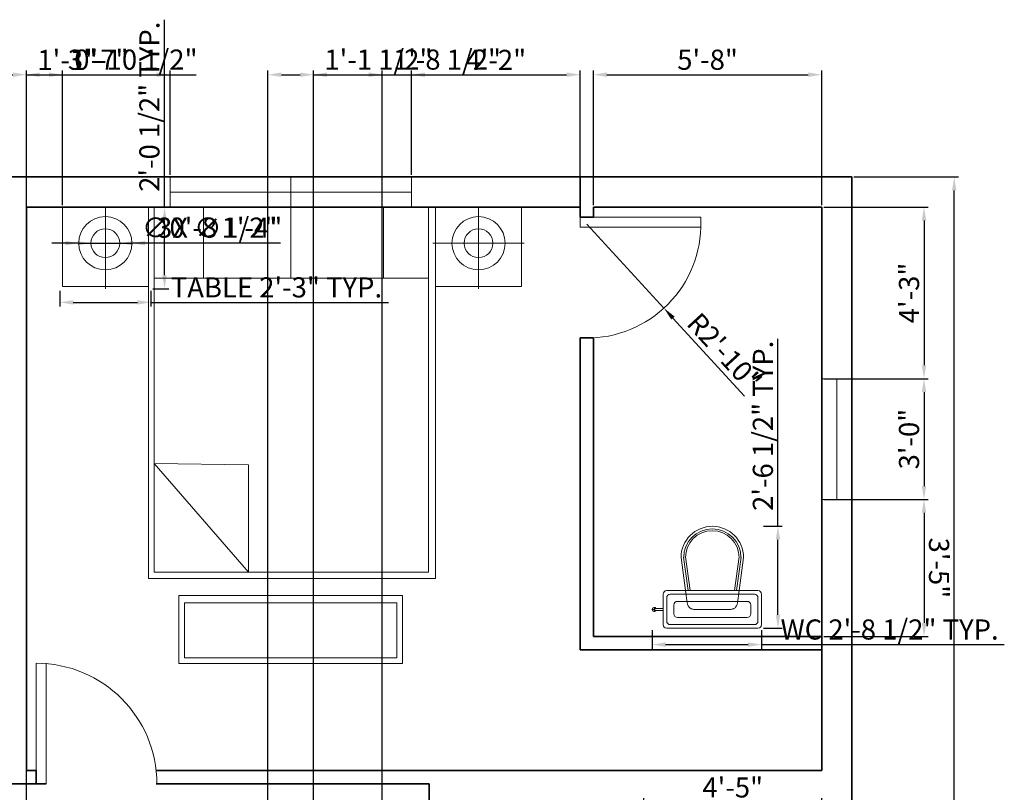
# Model space of a CAD drawing. Units: inches. Extents: x 1973 to 2661, y 1730 to 2412.
# Tile 5 of 5: x 2368 to 2661, y 2182 to 2412. Entities that reach past the tile are written whole.
import ezdxf

# ---------------------------------------------------------------- set-up
doc = ezdxf.new("R2010")
doc.units = ezdxf.units.IN
doc.linetypes.add('ACAD_ISO03W100', pattern=[30, 12, -18])
for name, color, linetype, lineweight in [('A-ANNO-DIMS', 2, 'Continuous', 18), ('A-DOOR', 3, 'Continuous', 18), ('A-FLOR-FIXT', 9, 'Continuous', 18), ('A-FLOR-FIXT-HIDN', 9, 'ACAD_ISO03W100', 13), ('A-FURN', 8, 'Continuous', 18), ('A-GLAZ', 4, 'Continuous', 18), ('A-WALL', 7, 'Continuous', 35)]:
    doc.layers.add(name, color=color, linetype=linetype, lineweight=lineweight)
doc.styles.get("Standard").update_dxf_attribs({"font": 'arial.ttf'})
doc.dimstyles.new('ISO-25', dxfattribs={"dimtxt": 6, "dimasz": 4, "dimexe": 1.25, "dimexo": 0.625, "dimtad": 1, "dimdec": 0, "dimrnd": 6, "dimlunit": 3, "dimtxsty": 'Standard', "dimcen": 2.5, "dimadec": 0, "dimazin": 0, "dimtfac": 1, "dimtdec": 0, "dimtmove": 0, "dimatfit": 3, "dimfxl": 1, "dimarcsym": 0})

# ---------------------------------------------------------------- blocks, each defined once
blk = doc.blocks.new('DOOR-36-SWING')
for p, q in [((0, 0), (0, 36)), ((0, 36), (0, 0)), ((3, 0), (3, 36)), ((0, 0), (3, 0))]:
    blk.add_line(p, q)
blk.add_arc((0, 0), 36, 0, 90)
blk = doc.blocks.new('WIN-72-TWO-LIGHT')
for p, q in [((0, 72), (9, 72)), ((0, 0), (0, 72)), ((4.5, 72), (4.5, 36)), ((9, 72), (9, 0)), ((4.5, 36), (0, 36)), ((0, 36), (9, 36)), ((4.5, 36), (4.5, 0)), ((9, 0), (0, 0))]:
    blk.add_line(p, q)
blk = doc.blocks.new('WC-TANK-PLAN')
for p, q in [((9.95, 11.2), (8.6, 21.07)), ((10.75, 11.2), (9.39, 21.19)), ((11.29, 11.2), (9.92, 21.26)), ((25.95, 21.26), (24.57, 11.2)), ((26.48, 21.19), (25.11, 11.2)), ((27.27, 21.07), (25.92, 11.2)), ((3.27, 1.07), (3.27, 10.13)), ((31.53, 11.2), (4.33, 11.2)), ((4.33, 2.13), (4.33, 9.07)), ((30.47, 10.13), (5.4, 10.13)), ((31.53, 2.13), (31.53, 9.07)), ((32.6, 1.07), (32.6, 10.13)), ((6.47, 4.27), (6.47, 6.93)), ((28.33, 8), (7.53, 8)), ((29.4, 4.27), (29.4, 6.93)), ((0.94, 5.6), (0.22, 5.6)), ((0.6, 5.33), (0.6, 5.87)), ((3.27, 5.87), (0.6, 5.87)), ((3.27, 5.33), (0.6, 5.33)), ((28.33, 3.2), (7.53, 3.2)), ((30.47, 1.07), (5.4, 1.07)), ((31.53, 0), (4.33, 0))]:
    blk.add_line(p, q)
for centre, radius, start, end in [((17.93, 21.07), 9.33, 0, 180), ((17.93, 21.07), 8.53, 0, 180), ((17.93, 21.07), 8, 0, 180), ((4.33, 10.13), 1.07, 90, 180), ((5.4, 9.07), 1.07, 90, 180), ((30.47, 9.07), 1.07, 0, 90), ((31.53, 10.13), 1.07, 0, 90), ((0.6, 5.6), 0.599, 26.4407, 333.5593), ((7.53, 6.93), 1.07, 90, 180), ((28.33, 6.93), 1.07, 0, 90), ((7.53, 4.27), 1.07, 180, 270), ((28.33, 4.27), 1.07, 270, 0), ((4.33, 1.07), 1.07, 180, 270), ((5.4, 2.13), 1.07, 180, 270), ((30.47, 2.13), 1.07, 270, 0), ((31.53, 1.07), 1.07, 270, 0)]:
    blk.add_arc(centre, radius, start, end)
blk = doc.blocks.new('BENCH-BED-END')
for p, q in [((0, 20.3), (0, 0)), ((66.64, 20.3), (0, 20.3)), ((1.73, 1.73), (1.73, 18.14)), ((1.73, 18.14), (64.92, 18.14)), ((64.92, 18.14), (64.92, 1.73)), ((66.64, 0), (66.64, 20.3)), ((64.92, 1.73), (1.73, 1.73)), ((0, 0), (66.64, 0))]:
    blk.add_line(p, q)
blk = doc.blocks.new('NIGHTSTAND-WITH-LAMP')
for p, q in [((0.77, 24.32), (0.77, 0.62)), ((13.58, 24.32, -15.39), (13.58, 0, -15.39)), ((27.15, 13.57, -15.39), (0, 13.57, -15.39)), ((0.77, 0.62), (26.42, 0.62))]:
    blk.add_line(p, q)
for radius in [7.93, 4.28]:
    blk.add_circle((13.58, 13.57, -15.39), radius)
blk = doc.blocks.new('*D22')
at = {"layer": 'A-ANNO-DIMS', "color": 0, "lineweight": -2, "transparency": 16777216}
for p, q in [((2556.52, 2230.17), (2556.52, 2224.65)), ((2589.12, 2230.17), (2589.12, 2224.65)), ((2560.52, 2225.9), (2585.12, 2225.9)), ((2589.12, 2225.9), (2661.47, 2225.9))]:
    blk.add_line(p, q, dxfattribs=at)
at = {"layer": 'A-ANNO-DIMS', "color": 0, "transparency": 16777216}
for points in [[(2560.52, 2226.57), (2560.52, 2225.24), (2556.52, 2225.9)], [(2585.12, 2226.57), (2585.12, 2225.24), (2589.12, 2225.9)]]:
    blk.add_solid(points, dxfattribs=at)
at = {"layer": 'Defpoints', "color": 0, "transparency": 16777216}
for p in [(2556.52, 2230.79), (2589.12, 2230.79), (2589.12, 2225.9)]:
    blk.add_point(p, dxfattribs=at)
at = {"layer": 'A-ANNO-DIMS', "color": 0, "transparency": 16777216, "insert": (2627.29, 2229.63), "char_height": 6, "attachment_point": 5}
blk.add_mtext('WC 2\'-8 1/2" TYP.', dxfattribs=at)
blk = doc.blocks.new('*D23')
at = {"layer": 'A-ANNO-DIMS', "color": 0, "lineweight": -2, "transparency": 16777216}
for p, q in [((2594.01, 2261.19), (2594.01, 2317.1)), ((2589.75, 2261.19), (2595.26, 2261.19)), ((2594.01, 2234.79), (2594.01, 2257.19)), ((2589.75, 2230.79), (2595.26, 2230.79))]:
    blk.add_line(p, q, dxfattribs=at)
at = {"layer": 'A-ANNO-DIMS', "color": 0, "transparency": 16777216}
for points in [[(2593.35, 2257.19), (2594.68, 2257.19), (2594.01, 2261.19)], [(2593.35, 2234.79), (2594.68, 2234.79), (2594.01, 2230.79)]]:
    blk.add_solid(points, dxfattribs=at)
at = {"layer": 'Defpoints', "color": 0, "transparency": 16777216}
for p in [(2589.12, 2261.19), (2594.01, 2261.19), (2589.12, 2230.79)]:
    blk.add_point(p, dxfattribs=at)
at = {"layer": 'A-ANNO-DIMS', "color": 0, "transparency": 16777216, "insert": (2590.29, 2291.15), "char_height": 6, "attachment_point": 5, "rotation": 90}
blk.add_mtext('2\'-6 1/2" TYP.', dxfattribs=at)
blk = doc.blocks.new('*D26')
at = {"layer": 'A-ANNO-DIMS', "color": 0, "lineweight": -2, "transparency": 16777216}
for p, q in [((2379.99, 2331.41), (2379.99, 2326.71)), ((2407.14, 2331.41), (2407.14, 2326.71)), ((2383.99, 2327.96), (2403.14, 2327.96)), ((2407.14, 2327.96), (2477.99, 2327.96))]:
    blk.add_line(p, q, dxfattribs=at)
at = {"layer": 'A-ANNO-DIMS', "color": 0, "transparency": 16777216}
for points in [[(2383.99, 2328.62), (2383.99, 2327.29), (2379.99, 2327.96)], [(2403.14, 2328.62), (2403.14, 2327.29), (2407.14, 2327.96)]]:
    blk.add_solid(points, dxfattribs=at)
at = {"layer": 'Defpoints', "color": 0, "transparency": 16777216}
for p in [(2379.99, 2332.03), (2407.14, 2332.03), (2407.14, 2327.96)]:
    blk.add_point(p, dxfattribs=at)
at = {"layer": 'A-ANNO-DIMS', "color": 0, "transparency": 16777216, "insert": (2444.56, 2331.65), "char_height": 6, "attachment_point": 5}
blk.add_mtext('TABLE 2\'-3" TYP.', dxfattribs=at)
blk = doc.blocks.new('*D27')
at = {"layer": 'A-ANNO-DIMS', "color": 0, "lineweight": -2, "transparency": 16777216}
for p, q in [((2411.21, 2356.35), (2411.21, 2412.26)), ((2407.76, 2356.35), (2412.46, 2356.35)), ((2411.21, 2336.03), (2411.21, 2352.35)), ((2407.76, 2332.03), (2412.46, 2332.03))]:
    blk.add_line(p, q, dxfattribs=at)
at = {"layer": 'A-ANNO-DIMS', "color": 0, "transparency": 16777216}
for points in [[(2410.54, 2352.35), (2411.87, 2352.35), (2411.21, 2356.35)], [(2410.54, 2336.03), (2411.87, 2336.03), (2411.21, 2332.03)]]:
    blk.add_solid(points, dxfattribs=at)
at = {"layer": 'Defpoints', "color": 0, "transparency": 16777216}
for p in [(2407.14, 2356.35), (2411.21, 2356.35), (2407.14, 2332.03)]:
    blk.add_point(p, dxfattribs=at)
at = {"layer": 'A-ANNO-DIMS', "color": 0, "transparency": 16777216, "insert": (2407.48, 2386.3), "char_height": 6, "attachment_point": 5, "rotation": 90}
blk.add_mtext('2\'-0 1/2" TYP.', dxfattribs=at)
blk = doc.blocks.new('*D31')
at = {"layer": 'A-ANNO-DIMS', "color": 0, "lineweight": -2, "transparency": 16777216}
for p, q in [((2616.67, 2365.35), (2647.79, 2365.35)), ((2646.54, 1769.35), (2646.54, 2361.35)), ((2616.67, 1765.35), (2647.79, 1765.35))]:
    blk.add_line(p, q, dxfattribs=at)
at = {"layer": 'A-ANNO-DIMS', "color": 0, "transparency": 16777216}
for points in [[(2645.88, 2361.35), (2647.21, 2361.35), (2646.54, 2365.35)], [(2645.88, 1769.35), (2647.21, 1769.35), (2646.54, 1765.35)]]:
    blk.add_solid(points, dxfattribs=at)
at = {"layer": 'Defpoints', "color": 0, "transparency": 16777216}
for p in [(2616.04, 2365.35), (2646.54, 2365.35), (2616.04, 1765.35)]:
    blk.add_point(p, dxfattribs=at)
at = {"layer": 'A-ANNO-DIMS', "color": 0, "transparency": 16777216, "insert": (2642.85, 2065.35), "char_height": 6, "attachment_point": 5, "rotation": 90}
blk.add_mtext('50\'-0"', dxfattribs=at)
blk = doc.blocks.new('*D37')
at = {"layer": 'A-ANNO-DIMS', "color": 0, "lineweight": -2, "transparency": 16777216}
for p, q in [((2370.04, 2356.98), (2370.04, 2397.1)), ((2374.04, 2395.85), (2408.84, 2395.85)), ((2412.84, 2365.96), (2412.84, 2397.1))]:
    blk.add_line(p, q, dxfattribs=at)
at = {"layer": 'A-ANNO-DIMS', "color": 0, "transparency": 16777216}
for points in [[(2374.04, 2396.52), (2374.04, 2395.18), (2370.04, 2395.85)], [(2408.84, 2396.52), (2408.84, 2395.18), (2412.84, 2395.85)]]:
    blk.add_solid(points, dxfattribs=at)
at = {"layer": 'Defpoints', "color": 0, "transparency": 16777216}
for p in [(2412.84, 2395.85), (2412.84, 2365.34), (2370.04, 2356.35)]:
    blk.add_point(p, dxfattribs=at)
at = {"layer": 'A-ANNO-DIMS', "color": 0, "transparency": 16777216, "insert": (2391.44, 2399.54), "char_height": 6, "attachment_point": 5}
blk.add_mtext('3\'-7"', dxfattribs=at)
blk = doc.blocks.new('*D38')
at = {"layer": 'A-ANNO-DIMS', "color": 0, "lineweight": -2, "transparency": 16777216}
for p, q in [((2484.84, 2365.96), (2484.84, 2397.1)), ((2488.84, 2395.85), (2531.04, 2395.85)), ((2535.04, 2356.98), (2535.04, 2397.1))]:
    blk.add_line(p, q, dxfattribs=at)
at = {"layer": 'A-ANNO-DIMS', "color": 0, "transparency": 16777216}
for points in [[(2488.84, 2396.52), (2488.84, 2395.18), (2484.84, 2395.85)], [(2531.04, 2396.52), (2531.04, 2395.18), (2535.04, 2395.85)]]:
    blk.add_solid(points, dxfattribs=at)
at = {"layer": 'Defpoints', "color": 0, "transparency": 16777216}
for p in [(2535.04, 2395.85), (2484.84, 2365.34), (2535.04, 2356.35)]:
    blk.add_point(p, dxfattribs=at)
at = {"layer": 'A-ANNO-DIMS', "color": 0, "transparency": 16777216, "insert": (2509.94, 2399.49), "char_height": 6, "attachment_point": 5}
blk.add_mtext('4\'-2"', dxfattribs=at)
blk = doc.blocks.new('*D39')
at = {"layer": 'A-ANNO-DIMS', "color": 0, "lineweight": -2, "transparency": 16777216}
for p, q in [((2539.04, 2356.98), (2539.04, 2397.1)), ((2543.04, 2395.85), (2603.04, 2395.85)), ((2607.04, 2356.98), (2607.04, 2397.1))]:
    blk.add_line(p, q, dxfattribs=at)
at = {"layer": 'A-ANNO-DIMS', "color": 0, "transparency": 16777216}
for points in [[(2543.04, 2396.52), (2543.04, 2395.18), (2539.04, 2395.85)], [(2603.04, 2396.52), (2603.04, 2395.18), (2607.04, 2395.85)]]:
    blk.add_solid(points, dxfattribs=at)
at = {"layer": 'Defpoints', "color": 0, "transparency": 16777216}
for p in [(2607.04, 2395.85), (2539.04, 2356.35), (2607.04, 2356.35)]:
    blk.add_point(p, dxfattribs=at)
at = {"layer": 'A-ANNO-DIMS', "color": 0, "transparency": 16777216, "insert": (2573.04, 2399.54), "char_height": 6, "attachment_point": 5}
blk.add_mtext('5\'-8"', dxfattribs=at)
blk = doc.blocks.new('*D50')
at = {"layer": 'A-ANNO-DIMS', "color": 0, "lineweight": -2, "transparency": 16777216}
for p, q in [((2607.66, 2269.19), (2638.79, 2269.2)), ((2637.54, 2265.2), (2637.54, 2232.36)), ((2607.67, 2228.35), (2638.79, 2228.36))]:
    blk.add_line(p, q, dxfattribs=at)
at = {"layer": 'A-ANNO-DIMS', "color": 0, "transparency": 16777216}
for points in [[(2638.2, 2265.2), (2636.87, 2265.2), (2637.54, 2269.2)], [(2638.21, 2232.36), (2636.88, 2232.36), (2637.54, 2228.36)]]:
    blk.add_solid(points, dxfattribs=at)
at = {"layer": 'Defpoints', "color": 0, "transparency": 16777216}
for p in [(2607.04, 2269.19), (2607.04, 2228.35), (2637.54, 2228.36)]:
    blk.add_point(p, dxfattribs=at)
at = {"layer": 'A-ANNO-DIMS', "color": 0, "transparency": 16777216, "insert": (2641.23, 2248.78), "char_height": 6, "attachment_point": 5, "rotation": 270.0074}
blk.add_mtext('3\'-5"', dxfattribs=at)
blk = doc.blocks.new('*D51')
at = {"layer": 'A-ANNO-DIMS', "color": 0, "lineweight": -2, "transparency": 16777216}
for p, q in [((2607.66, 2305.19), (2638.79, 2305.19)), ((2637.54, 2301.19), (2637.54, 2273.19)), ((2607.66, 2269.19), (2638.79, 2269.19))]:
    blk.add_line(p, q, dxfattribs=at)
at = {"layer": 'A-ANNO-DIMS', "color": 0, "transparency": 16777216}
for points in [[(2636.87, 2301.19), (2638.2, 2301.19), (2637.54, 2305.19)], [(2636.87, 2273.19), (2638.2, 2273.19), (2637.54, 2269.19)]]:
    blk.add_solid(points, dxfattribs=at)
at = {"layer": 'Defpoints', "color": 0, "transparency": 16777216}
for p in [(2607.04, 2305.19), (2607.04, 2269.19), (2637.54, 2269.19)]:
    blk.add_point(p, dxfattribs=at)
at = {"layer": 'A-ANNO-DIMS', "color": 0, "transparency": 16777216, "insert": (2633.85, 2287.19), "char_height": 6, "attachment_point": 5, "rotation": 90}
blk.add_mtext('3\'-0"', dxfattribs=at)
blk = doc.blocks.new('*D52')
at = {"layer": 'A-ANNO-DIMS', "color": 0, "lineweight": -2, "transparency": 16777216}
for p, q in [((2607.67, 2356.35), (2638.79, 2356.35)), ((2637.54, 2352.35), (2637.54, 2309.19)), ((2607.66, 2305.19), (2638.79, 2305.19))]:
    blk.add_line(p, q, dxfattribs=at)
at = {"layer": 'A-ANNO-DIMS', "color": 0, "transparency": 16777216}
for points in [[(2636.88, 2352.35), (2638.21, 2352.35), (2637.54, 2356.35)], [(2636.87, 2309.19), (2638.2, 2309.19), (2637.54, 2305.19)]]:
    blk.add_solid(points, dxfattribs=at)
at = {"layer": 'Defpoints', "color": 0, "transparency": 16777216}
for p in [(2607.04, 2356.35), (2607.04, 2305.19), (2637.54, 2305.19)]:
    blk.add_point(p, dxfattribs=at)
at = {"layer": 'A-ANNO-DIMS', "color": 0, "transparency": 16777216, "insert": (2633.85, 2330.77), "char_height": 6, "attachment_point": 5, "rotation": 89.9941}
blk.add_mtext('4\'-3"', dxfattribs=at)
blk = doc.blocks.new('*D63')
at = {"layer": 'A-ANNO-DIMS', "color": 0, "lineweight": -2, "transparency": 16777216}
for p, q in [((2554.04, 2148.98), (2554.04, 2180.1)), ((2558.04, 2178.85), (2603.04, 2178.85)), ((2607.04, 2148.98), (2607.04, 2180.1))]:
    blk.add_line(p, q, dxfattribs=at)
at = {"layer": 'A-ANNO-DIMS', "color": 0, "transparency": 16777216}
for points in [[(2558.04, 2179.52), (2558.04, 2178.18), (2554.04, 2178.85)], [(2603.04, 2179.52), (2603.04, 2178.18), (2607.04, 2178.85)]]:
    blk.add_solid(points, dxfattribs=at)
at = {"layer": 'Defpoints', "color": 0, "transparency": 16777216}
for p in [(2607.04, 2178.85), (2554.04, 2148.35), (2607.04, 2148.35)]:
    blk.add_point(p, dxfattribs=at)
at = {"layer": 'A-ANNO-DIMS', "color": 0, "transparency": 16777216, "insert": (2580.54, 2182.53), "char_height": 6, "attachment_point": 5}
blk.add_mtext('4\'-5"', dxfattribs=at)
blk = doc.blocks.new('*D67')
at = {"layer": 'A-ANNO-DIMS', "color": 0, "lineweight": -2, "transparency": 16777216}
for p, q in [((2455.64, 1843.98), (2455.64, 2397.1)), ((2459.64, 2395.85), (2472.06, 2395.85)), ((2476.06, 1843.98), (2476.06, 2397.1)), ((2476.06, 2395.85), (2510.68, 2395.85))]:
    blk.add_line(p, q, dxfattribs=at)
at = {"layer": 'A-ANNO-DIMS', "color": 0, "transparency": 16777216}
for points in [[(2459.64, 2396.52), (2459.64, 2395.18), (2455.64, 2395.85)], [(2472.06, 2396.52), (2472.06, 2395.18), (2476.06, 2395.85)]]:
    blk.add_solid(points, dxfattribs=at)
at = {"layer": 'Defpoints', "color": 0, "transparency": 16777216}
for p in [(2476.06, 2395.85), (2455.64, 1843.35), (2476.06, 1843.35)]:
    blk.add_point(p, dxfattribs=at)
at = {"layer": 'A-ANNO-DIMS', "color": 0, "transparency": 16777216, "insert": (2495.37, 2399.58), "char_height": 6, "attachment_point": 5}
blk.add_mtext('1\'-8 1/2"', dxfattribs=at)
blk = doc.blocks.new('*D68')
at = {"layer": 'A-ANNO-DIMS', "color": 0, "lineweight": -2, "transparency": 16777216}
for p, q in [((2442.04, 1843.98), (2442.04, 2397.1)), ((2446.04, 2395.85), (2451.64, 2395.85)), ((2455.64, 1843.98), (2455.64, 2397.1)), ((2455.64, 2395.85), (2490.26, 2395.85))]:
    blk.add_line(p, q, dxfattribs=at)
at = {"layer": 'A-ANNO-DIMS', "color": 0, "transparency": 16777216}
for points in [[(2446.04, 2396.52), (2446.04, 2395.18), (2442.04, 2395.85)], [(2451.64, 2396.52), (2451.64, 2395.18), (2455.64, 2395.85)]]:
    blk.add_solid(points, dxfattribs=at)
at = {"layer": 'Defpoints', "color": 0, "transparency": 16777216}
for p in [(2455.64, 2395.85), (2442.04, 1843.35), (2455.64, 1843.35)]:
    blk.add_point(p, dxfattribs=at)
at = {"layer": 'A-ANNO-DIMS', "color": 0, "transparency": 16777216, "insert": (2474.95, 2399.58), "char_height": 6, "attachment_point": 5}
blk.add_mtext('1\'-1 1/2"', dxfattribs=at)
blk = doc.blocks.new('*D69')
at = {"layer": 'A-ANNO-DIMS', "color": 0, "lineweight": -2, "transparency": 16777216}
for p, q in [((2357.02, 1843.98), (2357.02, 2397.1)), ((2361.02, 2395.85), (2366.04, 2395.85)), ((2370.04, 1843.98), (2370.04, 2397.1)), ((2370.04, 2395.85), (2390.68, 2395.85))]:
    blk.add_line(p, q, dxfattribs=at)
at = {"layer": 'A-ANNO-DIMS', "color": 0, "transparency": 16777216}
for points in [[(2361.02, 2396.52), (2361.02, 2395.18), (2357.02, 2395.85)], [(2366.04, 2396.52), (2366.04, 2395.18), (2370.04, 2395.85)]]:
    blk.add_solid(points, dxfattribs=at)
at = {"layer": 'Defpoints', "color": 0, "transparency": 16777216}
for p in [(2370.04, 2395.85), (2357.02, 1843.35), (2370.04, 1843.35)]:
    blk.add_point(p, dxfattribs=at)
at = {"layer": 'A-ANNO-DIMS', "color": 0, "transparency": 16777216, "insert": (2382.36, 2399.49), "char_height": 6, "attachment_point": 5}
blk.add_mtext('1\'-1"', dxfattribs=at)
blk = doc.blocks.new('*D82')
at = {"layer": 'A-ANNO-DIMS', "color": 0, "lineweight": -2, "transparency": 16777216}
for p, q in [((2370.04, 2356.98), (2370.04, 2397.1)), ((2374.04, 2395.85), (2376.75, 2395.85)), ((2380.75, 2356.98), (2380.75, 2397.1)), ((2380.75, 2395.85), (2420.59, 2395.85))]:
    blk.add_line(p, q, dxfattribs=at)
at = {"layer": 'A-ANNO-DIMS', "color": 0, "transparency": 16777216}
for points in [[(2374.04, 2396.52), (2374.04, 2395.18), (2370.04, 2395.85)], [(2376.75, 2396.52), (2376.75, 2395.18), (2380.75, 2395.85)]]:
    blk.add_solid(points, dxfattribs=at)
at = {"layer": 'Defpoints', "color": 0, "transparency": 16777216}
for p in [(2380.75, 2395.85), (2370.04, 2356.35), (2380.75, 2356.35)]:
    blk.add_point(p, dxfattribs=at)
at = {"layer": 'A-ANNO-DIMS', "color": 0, "transparency": 16777216, "insert": (2402.67, 2399.58), "char_height": 6, "attachment_point": 5}
blk.add_mtext('0\'-10 1/2"', dxfattribs=at)
blk = doc.blocks.new('*D84')
at = {"layer": 'A-ANNO-DIMS', "color": 0, "lineweight": -2, "transparency": 16777216}
for p, q in [((2537.04, 2351.31), (2560.03, 2326.23)), ((2584.08, 2299.99), (2562.73, 2323.28))]:
    blk.add_line(p, q, dxfattribs=at)
at = {"layer": 'A-ANNO-DIMS', "color": 0, "transparency": 16777216}
blk.add_solid([(2563.22, 2323.73), (2562.24, 2322.83), (2560.03, 2326.23)], dxfattribs=at)
at = {"layer": 'Defpoints', "color": 0, "transparency": 16777216}
for p in [(2537.04, 2351.31), (2560.03, 2326.23)]:
    blk.add_point(p, dxfattribs=at)
at = {"layer": 'A-ANNO-DIMS', "color": 0, "transparency": 16777216, "insert": (2577.48, 2312.65), "char_height": 6, "attachment_point": 5, "rotation": 312.5109}
blk.add_mtext('R2\'-10"', dxfattribs=at)
blk = doc.blocks.new('*D85')
at = {"layer": 'A-ANNO-DIMS', "color": 0, "lineweight": -2, "transparency": 16777216}
for p, q in [((2381.63, 2345.61), (2377.63, 2345.61)), ((2385.63, 2345.61), (2401.49, 2345.61)), ((2445.78, 2345.61), (2405.49, 2345.61))]:
    blk.add_line(p, q, dxfattribs=at)
at = {"layer": 'A-ANNO-DIMS', "color": 0, "transparency": 16777216}
for points in [[(2381.63, 2346.27), (2381.63, 2344.94), (2385.63, 2345.61)], [(2405.49, 2346.27), (2405.49, 2344.94), (2401.49, 2345.61)]]:
    blk.add_solid(points, dxfattribs=at)
at = {"layer": 'Defpoints', "color": 0, "transparency": 16777216}
for p in [(2385.63, 2345.61), (2401.49, 2345.61)]:
    blk.add_point(p, dxfattribs=at)
at = {"layer": 'A-ANNO-DIMS', "color": 0, "transparency": 16777216, "insert": (2427.63, 2349.46), "char_height": 6, "attachment_point": 5, "rotation": 0.0009}
blk.add_mtext('3X ∅1\'-4"', dxfattribs=at)
blk = doc.blocks.new('*D86')
at = {"layer": 'A-ANNO-DIMS', "color": 0, "lineweight": -2, "transparency": 16777216}
for p, q in [((2385.28, 2345.61), (2381.28, 2345.61)), ((2389.28, 2345.61), (2397.84, 2345.61)), ((2443.54, 2345.61), (2401.84, 2345.61))]:
    blk.add_line(p, q, dxfattribs=at)
at = {"layer": 'A-ANNO-DIMS', "color": 0, "transparency": 16777216}
for points in [[(2385.28, 2346.27), (2385.28, 2344.94), (2389.28, 2345.61)], [(2401.84, 2346.27), (2401.84, 2344.94), (2397.84, 2345.61)]]:
    blk.add_solid(points, dxfattribs=at)
at = {"layer": 'Defpoints', "color": 0, "transparency": 16777216}
for p in [(2389.28, 2345.61), (2397.84, 2345.61)]:
    blk.add_point(p, dxfattribs=at)
at = {"layer": 'A-ANNO-DIMS', "color": 0, "transparency": 16777216, "insert": (2424.69, 2349.46), "char_height": 6, "attachment_point": 5, "rotation": 0.0016}
blk.add_mtext('∅0\'-8 1/2"', dxfattribs=at)

msp = doc.modelspace()

# ---------------------------------------------------------------- linework, layer by layer
at = {"layer": 'A-DOOR'}
for p, q in [((2535.04, 2353.35), (2571.04, 2353.35)), ((2535.04, 2350.35), (2535.04, 2353.35)), ((2571.04, 2353.35), (2571.04, 2350.35)), ((2571.04, 2350.35), (2535.04, 2350.35))]:
    msp.add_line(p, q, dxfattribs=at)
msp.add_arc((2537.04, 2351.31), 34.01, 266.629, 358.3919, dxfattribs=at)
at = {"layer": 'A-FLOR-FIXT-HIDN'}
msp.add_lwpolyline([(2566.47, 2241.99), (2566.99, 2238.21, 0.371763), (2569.1, 2236.39), (2579.82, 2236.39, 0.371763), (2581.93, 2238.21), (2582.44, 2241.99)], format="xyb", dxfattribs=at)
at = {"layer": 'A-FURN'}
for p, q in [((2406.41, 2245.64), (2406.41, 2356.35)), ((2408.13, 2356.34), (2489.89, 2356.34)), ((2408.13, 2247.48), (2408.13, 2356.34)), ((2422.81, 2356.34), (2422.81, 2335.17)), ((2448.84, 2356.34), (2448.84, 2335.17)), ((2476.5, 2356.34), (2476.5, 2335.17)), ((2489.89, 2356.34), (2489.89, 2247.48)), ((2491.94, 2356.35), (2491.94, 2245.64)), ((2489.89, 2335.17), (2408.13, 2335.17)), ((2436.19, 2279.55), (2408.13, 2279.88)), ((2408.13, 2279.88), (2436.19, 2247.48)), ((2436.19, 2247.48), (2436.19, 2279.55)), ((2491.94, 2245.64), (2406.41, 2245.64)), ((2489.89, 2247.48), (2408.13, 2247.48))]:
    msp.add_line(p, q, dxfattribs=at)
at = {"layer": 'A-GLAZ'}
for p, q in [((2607.04, 2269.19), (2607.04, 2305.19)), ((2607.04, 2305.19), (2616.04, 2305.19)), ((2611.54, 2269.19), (2611.54, 2305.19)), ((2616.04, 2305.19), (2616.04, 2269.19)), ((2616.04, 2269.19), (2607.04, 2269.19)), ((2607.04, 2269.19), (2611.54, 2269.19))]:
    msp.add_line(p, q, dxfattribs=at)
at = {"layer": 'A-WALL'}
for p, q in [((2016.04, 2365.35), (2616.04, 2365.35)), ((2535.04, 2365.35), (2535.04, 2353.35)), ((2616.04, 2365.35), (2616.04, 1765.35)), ((2535.04, 2356.35), (2370.04, 2356.35)), ((2370.04, 2356.35), (2370.04, 2188.35)), ((2539.04, 2353.35), (2539.04, 2356.35)), ((2539.04, 2356.35), (2607.04, 2356.35)), ((2607.04, 2356.35), (2607.04, 2188.35)), ((2535.04, 2353.35), (2539.04, 2353.35)), ((2535.04, 2317.35), (2539.04, 2317.35)), ((2535.04, 2224.35), (2535.04, 2317.35)), ((2539.04, 2317.35), (2539.04, 2228.35)), ((2539.04, 2228.35), (2607.04, 2228.35)), ((2607.04, 2224.35), (2535.04, 2224.35)), ((2370.04, 2188.35), (2372.94, 2188.35)), ((2370.04, 2188.35), (2372.94, 2188.35)), ((2372.94, 2188.35), (2372.94, 2184.35)), ((2607.04, 2188.35), (2408.72, 2188.35)), ((2237.06, 2184.35), (2375.94, 2184.35)), ((2408.72, 2184.35), (2490.04, 2184.35)), ((2490.04, 2184.35), (2490.04, 1843.35))]:
    msp.add_line(p, q, dxfattribs=at)

# ---------------------------------------------------------------- block references
at = {"layer": 'A-DOOR'}
msp.add_blockref('DOOR-36-SWING', (2372.94, 2184.35), dxfattribs=at)
at = {"layer": 'A-FLOR-FIXT'}
msp.add_blockref('WC-TANK-PLAN', (2556.52, 2230.79), dxfattribs=at)
at = {"layer": 'A-FURN'}
for name, p in [('NIGHTSTAND-WITH-LAMP', (2379.99, 2332.03)), ('BENCH-BED-END', (2415.47, 2220.26))]:
    msp.add_blockref(name, p, dxfattribs=at)
at = {"layer": 'A-FURN', "extrusion": (0, 0, -1), "zscale": -1}
msp.add_blockref('NIGHTSTAND-WITH-LAMP', (-2518.36, 2332.03), dxfattribs=at)
at = {"layer": 'A-GLAZ', "rotation": 270.0000000000011}
msp.add_blockref('WIN-72-TWO-LIGHT', (2412.84, 2365.34), dxfattribs=at)

# ---------------------------------------------------------------- dimensions: what is measured, and where the dimension line sits
at = {"layer": 'A-ANNO-DIMS'}
for base, p1, p2, picture, middle in [((2411.21, 2356.35), (2407.14, 2332.03), (2407.14, 2356.35), '*D27', (2407.48, 2386.3)), ((2594.01, 2261.19), (2589.12, 2230.79), (2589.12, 2261.19), '*D23', (2590.29, 2291.15))]:
    dim = msp.add_linear_dim(base=base, p1=p1, p2=p2, angle=90, text='<> TYP.', dimstyle='ISO-25', override={"dimdec": 1, "dimlfac": 1, "dimrnd": 0, "dimzin": 1, "dimdsep": 46, "dimlunit": 4, "dimfrac": 2}, dxfattribs=at)
    dim.commit()
    dim.dimension.update_dxf_attribs({"geometry": picture, "text_midpoint": middle})
for base, p1, p2, picture, middle in [((2380.75, 2395.85), (2370.04, 2356.35), (2380.75, 2356.35), '*D82', (2402.67, 2399.58)), ((2455.64, 2395.85), (2442.04, 1843.35), (2455.64, 1843.35), '*D68', (2474.95, 2399.58)), ((2476.06, 2395.85), (2455.64, 1843.35), (2476.06, 1843.35), '*D67', (2495.37, 2399.58)), ((2370.04, 2395.85), (2357.02, 1843.35), (2370.04, 1843.35), '*D69', (2382.36, 2399.49)), ((2412.84, 2395.85), (2370.04, 2356.35), (2412.84, 2365.34), '*D37', (2391.44, 2399.54)), ((2535.04, 2395.85), (2484.84, 2365.34), (2535.04, 2356.35), '*D38', (2509.94, 2399.49)), ((2607.04, 2395.85), (2539.04, 2356.35), (2607.04, 2356.35), '*D39', (2573.04, 2399.54)), ((2607.04, 2178.85), (2554.04, 2148.35), (2607.04, 2148.35), '*D63', (2580.54, 2182.53))]:
    dim = msp.add_linear_dim(base=base, p1=p1, p2=p2, dimstyle='ISO-25', override={"dimdec": 1, "dimlfac": 1, "dimrnd": 0, "dimzin": 1, "dimdsep": 46, "dimlunit": 4, "dimfrac": 2}, dxfattribs=at)
    dim.commit()
    dim.dimension.update_dxf_attribs({"geometry": picture, "text_midpoint": middle})
for base, p1, p2, angle, picture, middle in [((2646.54, 2365.35), (2616.04, 1765.35), (2616.04, 2365.35), 90, '*D31', (2642.85, 2065.35)), ((2637.54, 2305.19), (2607.04, 2356.35), (2607.04, 2305.19), 269.9941, '*D52', (2633.85, 2330.77)), ((2637.54, 2269.19), (2607.04, 2305.19), (2607.04, 2269.19), 270, '*D51', (2633.85, 2287.19)), ((2637.54, 2228.36), (2607.04, 2269.19), (2607.04, 2228.35), 270.0074, '*D50', (2641.23, 2248.78))]:
    dim = msp.add_linear_dim(base=base, p1=p1, p2=p2, angle=angle, dimstyle='ISO-25', override={"dimdec": 1, "dimlfac": 1, "dimrnd": 0, "dimzin": 1, "dimdsep": 46, "dimlunit": 4, "dimfrac": 2}, dxfattribs=at)
    dim.commit()
    dim.dimension.update_dxf_attribs({"geometry": picture, "text_midpoint": middle})
dim = msp.add_diameter_dim_2p(p1=(2385.63, 2345.61), p2=(2401.49, 2345.61), text='3X <>', dimstyle='ISO-25', override={"dimdec": 1, "dimlfac": 1, "dimrnd": 0, "dimzin": 1, "dimdsep": 46, "dimlunit": 4, "dimfrac": 2}, dxfattribs=at)
dim.commit()
dim.dimension.update_dxf_attribs({"geometry": '*D85', "text_midpoint": (2427.63, 2345.61)})
dim = msp.add_diameter_dim_2p(p1=(2389.28, 2345.61), p2=(2397.84, 2345.61), dimstyle='ISO-25', override={"dimdec": 1, "dimlfac": 1, "dimrnd": 0, "dimzin": 1, "dimdsep": 46, "dimlunit": 4, "dimfrac": 2}, dxfattribs=at)
dim.commit()
dim.dimension.update_dxf_attribs({"geometry": '*D86', "text_midpoint": (2424.69, 2345.61)})
dim = msp.add_radius_dim(center=(2537.04, 2351.31), mpoint=(2560.03, 2326.23), dimstyle='ISO-25', override={"dimdec": 1, "dimlfac": 1, "dimrnd": 0, "dimzin": 1, "dimdsep": 46, "dimlunit": 4, "dimfrac": 2}, dxfattribs=at)
dim.commit()
dim.dimension.update_dxf_attribs({"geometry": '*D84', "text_midpoint": (2577.48, 2312.65)})
for base, p1, p2, text, picture, middle in [((2407.1356, 2327.958), (2379.985, 2332.0306), (2407.1356, 2332.0306), 'TABLE <> TYP.', '*D26', (2444.5641, 2331.6485)), ((2589.12, 2225.9), (2556.52, 2230.79), (2589.12, 2230.79), 'WC <> TYP.', '*D22', (2627.29, 2229.63))]:
    dim = msp.add_linear_dim(base=base, p1=p1, p2=p2, text=text, dimstyle='ISO-25', override={"dimdec": 1, "dimlfac": 1, "dimrnd": 0, "dimzin": 1, "dimdsep": 46, "dimlunit": 4, "dimfrac": 2}, dxfattribs=at)
    dim.commit()
    dim.dimension.update_dxf_attribs({"geometry": picture, "text_midpoint": middle})

doc.saveas('drawing.dxf')
